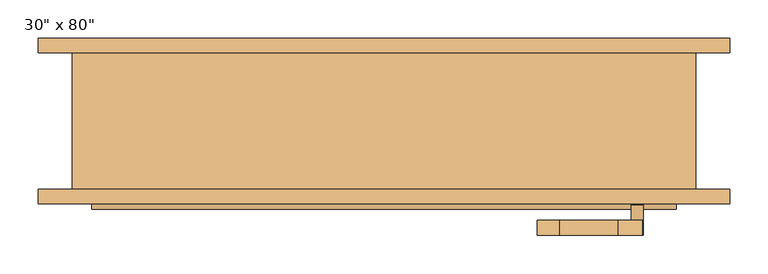
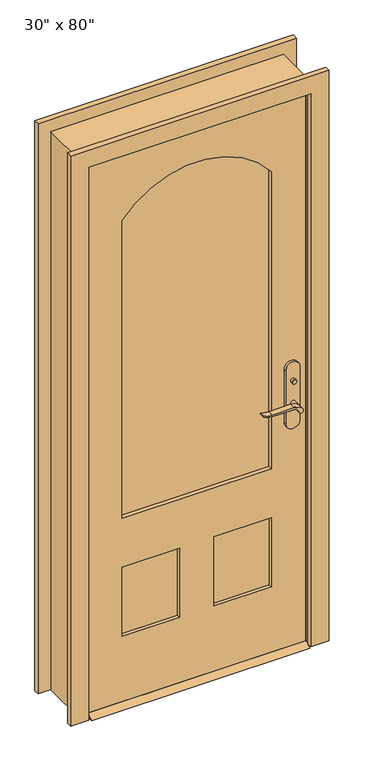
"""IFC4 building model written with IfcOpenShell, lengths in millimetres: door geometry."""

from ifc_helpers import new_model, si_unit, point, frame, frame_2d, origin, place, context, project, spatial, polyline, circle_curve, trimmed, segment, composite_curve, outline, extrude, faceted_brep, source, transform, mapped, element, save


def door_195c67e9(model_context):
    return source(origin(), model_context, "Body", "SolidModel", [
        extrude(outline(polyline([(-50.8, 12.7), (-25.4, 0.0), (-111.125, 0.0), (-85.725, 12.7), (-50.8, 12.7)])), frame((-381.0, 0.0, 0.0), z_axis=(1.0, 0.0, 0.0), x_axis=(0.0, 1.0, 0.0)), (0.0, 0.0, 1.0), 762.0),
        extrude(outline(polyline([(335.2, -30.8), (335.2, -40.8), (325.2, -40.8), (325.2, -30.8), (335.2, -30.8)])), frame((0.0, 0.0, 981.9), z_axis=(0.0, 0.0, 1.0), x_axis=(1.0, 0.0, 0.0)), (0.0, 0.0, 1.0), 30.0),
        extrude(outline(composite_curve([segment(trimmed(circle_curve(frame_2d((996.9, 330.2)), 8.0), [point((996.9, 322.2))], [point((996.9, 338.2))], False, "CARTESIAN"), True, "CONTINUOUS"), segment(trimmed(circle_curve(frame_2d((996.9, 330.2)), 8.0), [point((996.9, 338.2))], [point((996.9, 322.2))], False, "CARTESIAN"), True, "CONTINUOUS")], self_intersect=False)), frame((0.0, -105.725, 0.0), z_axis=(0.0, 1.0, 0.0), x_axis=(0.0, 0.0, 1.0)), (0.0, 0.0, 1.0), 10.0),
        extrude(outline(composite_curve([segment(trimmed(circle_curve(frame_2d((897.1555521, 306.5324871)), 37.2832219), [point((919.0523287, 336.7081363))], [point((934.4, 304.8325667))], False, "CARTESIAN"), True, "CONTINUOUS"), segment(polyline([(934.4, 304.8325667), (934.4, 228.5564091)]), True, "CONTINUOUS"), segment(trimmed(circle_curve(frame_2d((1017.6850638, 228.6227909)), 83.2850902), [point((934.4, 228.5564091))], [point((939.4, 200.2))], True, "CARTESIAN"), True, "CONTINUOUS"), segment(polyline([(939.4, 200.2), (936.6135558, 200.2)]), True, "CONTINUOUS"), segment(trimmed(circle_curve(frame_2d((986.6709207, 232.1396612)), 59.3791355), [point((936.6135558, 200.2))], [point((927.4, 228.5564091))], False, "CARTESIAN"), True, "CONTINUOUS"), segment(polyline([(927.4, 228.5564091), (927.4, 304.8138099)]), True, "CONTINUOUS"), segment(trimmed(circle_curve(frame_2d((909.2738613, 304.8138099)), 18.1261387), [point((927.4, 304.8138099))], [point((914.4, 322.2))], True, "CARTESIAN"), True, "CONTINUOUS"), segment(trimmed(circle_curve(frame_2d((914.4, 330.2)), 8.0), [point((914.4, 322.2))], [point((919.0523287, 336.7081363))], False, "CARTESIAN"), True, "CONTINUOUS")], self_intersect=False)), frame((0.0, -10.8, 0.0), z_axis=(0.0, 1.0, 0.0), x_axis=(0.0, 0.0, 1.0)), (0.0, 0.0, 1.0), 20.0),
        extrude(outline(composite_curve([segment(trimmed(circle_curve(frame_2d((914.4, 330.2)), 8.0), [point((914.3999903, 322.2))], [point((919.0523287, 336.7081363))], False, "CARTESIAN"), True, "CONTINUOUS"), segment(trimmed(circle_curve(frame_2d((897.1555521, 306.5324871)), 37.2832219), [point((919.0523287, 336.7081363))], [point((934.4, 304.8325667))], False, "CARTESIAN"), True, "CONTINUOUS"), segment(polyline([(934.4, 304.8325667), (934.4, 228.5564091)]), True, "CONTINUOUS"), segment(trimmed(circle_curve(frame_2d((1017.6850638, 228.6227909)), 83.2850902), [point((934.4, 228.5564091))], [point((939.4, 200.2))], True, "CARTESIAN"), True, "CONTINUOUS"), segment(polyline([(939.4, 200.2), (936.6135558, 200.2)]), True, "CONTINUOUS"), segment(trimmed(circle_curve(frame_2d((986.6709207, 232.1396612)), 59.3791355), [point((936.6135558, 200.2))], [point((927.4, 228.5564091))], False, "CARTESIAN"), True, "CONTINUOUS"), segment(polyline([(927.4, 228.5564091), (927.4, 304.8138122)]), True, "CONTINUOUS"), segment(trimmed(circle_curve(frame_2d((909.2738682, 304.8138122)), 18.1261318), [point((927.4, 304.8138122))], [point((914.3999903, 322.2))], True, "CARTESIAN"), True, "CONTINUOUS")], self_intersect=False)), frame((0.0, -145.725, 0.0), z_axis=(0.0, 1.0, 0.0), x_axis=(0.0, 0.0, 1.0)), (0.0, 0.0, 1.0), 20.0),
        extrude(outline(composite_curve([segment(trimmed(circle_curve(frame_2d((914.4, 330.2)), 8.0), [point((914.4, 322.2))], [point((914.4, 338.2))], False, "CARTESIAN"), True, "CONTINUOUS"), segment(trimmed(circle_curve(frame_2d((914.4, 330.2)), 8.0), [point((914.4, 338.2))], [point((914.4, 322.2))], False, "CARTESIAN"), True, "CONTINUOUS")], self_intersect=False)), frame((0.0, -40.8, 0.0), z_axis=(0.0, 1.0, 0.0), x_axis=(0.0, 0.0, 1.0)), (0.0, 0.0, 1.0), 30.0),
        extrude(outline(composite_curve([segment(trimmed(circle_curve(frame_2d((914.4, 330.2)), 8.0), [point((914.4, 322.2))], [point((914.4, 338.2))], False, "CARTESIAN"), True, "CONTINUOUS"), segment(trimmed(circle_curve(frame_2d((914.4, 330.2)), 8.0), [point((914.4, 338.2))], [point((914.4, 322.2))], False, "CARTESIAN"), True, "CONTINUOUS")], self_intersect=False)), frame((0.0, -125.725, 0.0), z_axis=(0.0, 1.0, 0.0), x_axis=(0.0, 0.0, 1.0)), (0.0, 0.0, 1.0), 30.0),
        extrude(outline(composite_curve([segment(polyline([(844.4, 355.2), (1039.4, 355.2)]), True, "CONTINUOUS"), segment(trimmed(circle_curve(frame_2d((1039.4, 330.2)), 25.0), [point((1039.4, 355.2))], [point((1039.4, 305.2))], False, "CARTESIAN"), True, "CONTINUOUS"), segment(polyline([(1039.4, 305.2), (844.4, 305.2)]), True, "CONTINUOUS"), segment(trimmed(circle_curve(frame_2d((844.4, 330.2)), 25.0), [point((844.4, 305.2))], [point((844.4, 355.2))], False, "CARTESIAN"), True, "CONTINUOUS")], self_intersect=False)), frame((0.0, -50.8, 0.0), z_axis=(0.0, 1.0, 0.0), x_axis=(0.0, 0.0, 1.0)), (0.0, 0.0, 1.0), 10.0),
        extrude(outline(composite_curve([segment(polyline([(844.4, 355.2), (1039.4, 355.2)]), True, "CONTINUOUS"), segment(trimmed(circle_curve(frame_2d((1039.4, 330.2)), 25.0), [point((1039.4, 355.2))], [point((1039.4, 305.2))], False, "CARTESIAN"), True, "CONTINUOUS"), segment(polyline([(1039.4, 305.2), (844.4, 305.2)]), True, "CONTINUOUS"), segment(trimmed(circle_curve(frame_2d((844.4, 330.2)), 25.0), [point((844.4, 305.2))], [point((844.4, 355.2))], False, "CARTESIAN"), True, "CONTINUOUS")], self_intersect=False)), frame((0.0, -95.725, 0.0), z_axis=(0.0, 1.0, 0.0), x_axis=(0.0, 0.0, 1.0)), (0.0, 0.0, 1.0), 10.0),
        extrude(outline(polyline([(2032.0, -381.0), (12.7, -381.0), (12.7, 381.0), (2032.0, 381.0), (2032.0, -381.0)]), holes=[composite_curve([segment(polyline([(688.975, -260.35), (1784.35, -260.35)]), True, "CONTINUOUS"), segment(trimmed(circle_curve(frame_2d((1580.99125, 0.0)), 330.35875), [point((1784.35, -260.35))], [point((1784.35, 260.35))], True, "CARTESIAN"), True, "CONTINUOUS"), segment(polyline([(1784.35, 260.35), (688.975, 260.35), (688.975, -260.35)]), True, "CONTINUOUS")], self_intersect=False), polyline([(508.0, -60.325), (254.0, -60.325), (254.0, -260.35), (508.0, -260.35), (508.0, -60.325)]), polyline([(508.0, 260.35), (254.0, 260.35), (254.0, 60.325), (508.0, 60.325), (508.0, 260.35)])]), frame((0.0, -85.725, 0.0), z_axis=(0.0, 1.0, 0.0), x_axis=(0.0, 0.0, 1.0)), (0.0, 0.0, 1.0), 34.925),
        faceted_brep([(406.4, -85.725, 0.0), (381.0, -85.725, 0.0), (381.0, -50.8, 0.0), (368.3, -50.8, 0.0), (368.3, -15.875, 0.0), (381.0, -15.875, 0.0), (381.0, 92.075, 0.0), (406.4, 92.075, 0.0), (406.4, 92.075, 2057.4), (406.4, -85.725, 2057.4), (381.0, 92.075, 2032.0), (-381.0, 92.075, 2032.0), (-381.0, 92.075, 0.0), (-406.4, 92.075, 0.0), (-406.4, 92.075, 2057.4), (381.0, -15.875, 2032.0), (368.3, -15.875, 2019.3), (-368.3, -15.875, 2019.3), (-368.3, -15.875, 0.0), (-381.0, -15.875, 0.0), (-381.0, -15.875, 2032.0), (368.3, -50.8, 2019.3), (381.0, -50.8, 2032.0), (-381.0, -50.8, 2032.0), (-381.0, -50.8, 0.0), (-368.3, -50.8, 0.0), (-368.3, -50.8, 2019.3), (381.0, -85.725, 2032.0), (-406.4, -85.725, 2057.4), (-406.4, -85.725, 0.0), (-381.0, -85.725, 0.0), (-381.0, -85.725, 2032.0)], [[[0, 1, 2, 3, 4, 5, 6, 7]], [[7, 8, 9, 0]], [[6, 10, 11, 12, 13, 14, 8, 7]], [[5, 15, 10, 6]], [[4, 16, 17, 18, 19, 20, 15, 5]], [[3, 21, 16, 4]], [[2, 22, 23, 24, 25, 26, 21, 3]], [[1, 27, 22, 2]], [[0, 9, 28, 29, 30, 31, 27, 1]], [[8, 14, 28, 9]], [[15, 20, 11, 10]], [[21, 26, 17, 16]], [[27, 31, 23, 22]], [[29, 13, 12, 19, 18, 25, 24, 30]], [[14, 13, 29, 28]], [[20, 19, 12, 11]], [[26, 25, 18, 17]], [[31, 30, 24, 23]]]),
        extrude(outline(polyline([(-60.325, -62.4416667), (-60.325, -74.0833333), (-260.35, -74.0833333), (-260.35, -62.4416667), (-60.325, -62.4416667)])), frame((0.0, 0.0, 254.0), z_axis=(0.0, 0.0, 1.0), x_axis=(1.0, 0.0, 0.0)), (0.0, 0.0, 1.0), 254.0),
        extrude(outline(polyline([(260.35, -62.4416667), (260.35, -74.0833333), (60.325, -74.0833333), (60.325, -62.4416667), (260.35, -62.4416667)])), frame((0.0, 0.0, 254.0), z_axis=(0.0, 0.0, 1.0), x_axis=(1.0, 0.0, 0.0)), (0.0, 0.0, 1.0), 254.0),
        extrude(outline(composite_curve([segment(polyline([(688.975, -260.35), (688.975, 260.35), (1784.35, 260.35)]), True, "CONTINUOUS"), segment(trimmed(circle_curve(frame_2d((1580.99125, 0.0)), 330.35875), [point((1784.35, 260.35))], [point((1784.35, -260.35))], False, "CARTESIAN"), True, "CONTINUOUS"), segment(polyline([(1784.35, -260.35), (688.975, -260.35)]), True, "CONTINUOUS")], self_intersect=False)), frame((0.0, -71.755, 0.0), z_axis=(0.0, 1.0, 0.0), x_axis=(0.0, 0.0, 1.0)), (0.0, 0.0, 1.0), 6.985),
        extrude(outline(polyline([(0.0, -387.35), (2038.35, -387.35), (2038.35, 387.35), (0.0, 387.35), (0.0, 450.85), (2101.85, 450.85), (2101.85, -450.85), (0.0, -450.85), (0.0, -387.35)])), frame((0.0, 92.075, 0.0), z_axis=(0.0, 1.0, 0.0), x_axis=(0.0, 0.0, 1.0)), (0.0, 0.0, 1.0), 19.05),
        extrude(outline(polyline([(0.0, -387.35), (2038.35, -387.35), (2038.35, 387.35), (0.0, 387.35), (0.0, 450.85), (2101.85, 450.85), (2101.85, -450.85), (0.0, -450.85), (0.0, -387.35)])), frame((0.0, -104.775, 0.0), z_axis=(0.0, 1.0, 0.0), x_axis=(0.0, 0.0, 1.0)), (0.0, 0.0, 1.0), 19.05),
    ])


if __name__ == "__main__":
    model = new_model("IFC4")
    model_context = context("Model", 3, world=origin())
    ifc_project = project(units=[si_unit("LENGTHUNIT", "METRE", prefix="MILLI")], contexts=[model_context])
    site = spatial("IfcSite", under=ifc_project)
    building = spatial("IfcBuilding", under=site)
    placement = place(None, origin())
    door_shape = door_195c67e9(model_context)
    element("IfcDoor", 1, ObjectType="30\" x 80\"", at=placement, inside=building, context=model_context, shape_type="MappedRepresentation", body=[
        mapped(door_shape, transform((0.0, 0.0, 0.0), x_axis=(1.0, 0.0, 0.0), y_axis=(0.0, 1.0, 0.0), z_axis=(0.0, 0.0, 1.0))),
    ])
    save(model, "model.ifc")

# Revit data of these elements
# Type "30\" x 80\""
#   Type Mark = "9"
#   Assembly Code = "B2030100"
#   Analytic Construction = "French door, wood frame with single glass"
#   Threshold Offset [instance default] = 0' - 0 1/2"
#   Thickness = 0' - 1 3/8"
#   Thermal Resistance (R) = 1.0696 (h·ft²·°F)/BTU
#   Swing Angle [instance default] = 90.00°
#   Stiles = 0' - 4 3/4"
#   Rough Width = 2' - 8"
#   Rough Height = 6' - 9"
#   Radius = 1' - 1.00625"
#   Lock Rail = 0' - 7 1/8"
#   Height = 6' - 8"
#   Width = 2' - 6"
#   Heat Transfer Coefficient (U) = 0.9350 BTU/(h·ft²·°F)
#   Door Offset [instance default] = 0' - 0"
#   Bottom Rail = 0' - 9 1/2"
#   Threshold [instance default] = yes
#   Function = 1
#   Exterior Trim [instance default] = yes
#   Trim Material = Cherry
#   Threshold Material = Cherry
#   Panel Material = Cherry
#   Glazing = Glass
#   Frame Material = Cherry
#   Door Handle Material = Aluminum
#   Visual Light Transmittance = 0
#   Solar Heat Gain Coefficient = 0
#   Wall Closure = (empty or 0)
#   Construction Type = (empty or 0)
# Element 1 (IfcDoor, "30\" x 80\"")
#   Materials on its faces: "Cherry", "Aluminum", "Glass"
# Materials
#   "Cherry": class "Wood", colour RGB 226 177 128, transparency 0, Description = "Prunus Serotina", Cost = 0
#   "Glass": class "Glass", colour RGB 0 128 192, transparency 0.75, Description = "Soda Lime Glass", Cost = 0
#   "Aluminum": class "Metal", colour RGB 247 247 247, transparency 0, Description = "Aluminum 6061", Cost = 0
